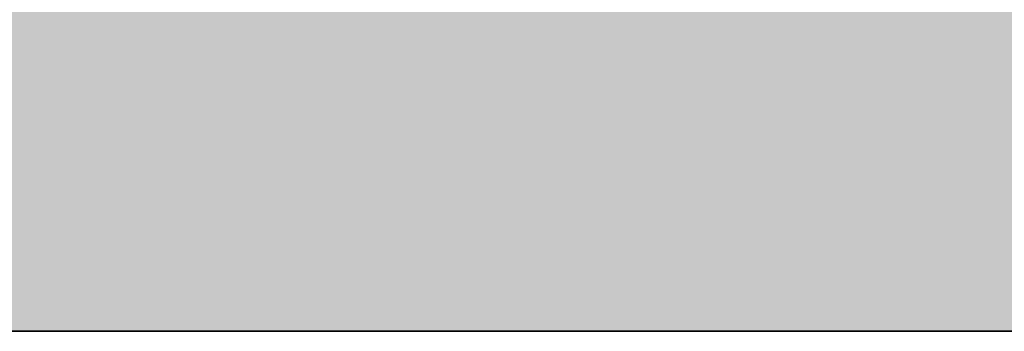
# Model space of a CAD drawing. Units: inches. Extents: x 2083 to 3317, y 1141 to 2115.
# Tile 141 of 256: x 3126.6699 to 3126.8176, y 1263.2614 to 1263.3081. Entities that reach past the tile are written whole.
import ezdxf

# ---------------------------------------------------------------- set-up
doc = ezdxf.new("R2010")
doc.units = ezdxf.units.IN
doc.layers.add('A-ANNO-DIMS', color=2, linetype='Continuous', lineweight=18)
doc.layers.add('A-WALL', color=7, linetype='Continuous', lineweight=35)
doc.layers.add('A-WALL-PATT', color=251, linetype='Continuous', lineweight=13, true_color=0x636466)
doc.styles.get("Standard").update_dxf_attribs({"font": 'arial.ttf'})
doc.dimstyles.new('ISO-25', dxfattribs={"dimtxt": 12, "dimasz": 12, "dimexe": 1.25, "dimexo": 0.625, "dimtad": 1, "dimlunit": 3, "dimtxsty": 'Standard', "dimcen": 2.5, "dimadec": 0, "dimazin": 0, "dimtfac": 1, "dimtmove": 0, "dimatfit": 3, "dimfxl": 1, "dimarcsym": 0})

# ---------------------------------------------------------------- blocks, each defined once
blk = doc.blocks.new('*D10')
at = {"layer": 'A-ANNO-DIMS', "color": 0, "lineweight": -2, "transparency": 16777216}
for p, q in [((2862.95978, 1262.63636), (2862.95978, 1201.38445)), ((3126.95978, 1262.63636), (3126.95978, 1201.38445)), ((2874.95978, 1202.63445), (3114.95978, 1202.63445))]:
    blk.add_line(p, q, dxfattribs=at)
at = {"layer": 'A-ANNO-DIMS', "color": 0, "transparency": 16777216}
for points in [[(2874.95978, 1204.63445), (2874.95978, 1200.63445), (2862.95978, 1202.63445)], [(3114.95978, 1204.63445), (3114.95978, 1200.63445), (3126.95978, 1202.63445)]]:
    blk.add_solid(points, dxfattribs=at)
at = {"layer": 'Defpoints', "color": 0, "transparency": 16777216}
for p in [(2862.95978, 1263.26136), (3126.95978, 1263.26136), (3126.95978, 1202.63445)]:
    blk.add_point(p, dxfattribs=at)
at = {"layer": 'A-ANNO-DIMS', "color": 0, "transparency": 16777216, "insert": (2994.95978, 1209.28401), "char_height": 12, "attachment_point": 5}
blk.add_mtext("22'", dxfattribs=at)
blk = doc.blocks.new('*D26')
at = {"layer": 'A-ANNO-DIMS', "color": 0, "lineweight": -2, "transparency": 16777216}
for p, q in [((3088.98584, 1274.91509), (3088.98584, 1270.95196)), ((3111.24004, 1274.91509), (3111.24004, 1270.95196)), ((3076.98584, 1272.20196), (2840.26245, 1272.20196)), ((3111.24004, 1272.20196), (3088.98584, 1272.20196)), ((3123.24004, 1272.20196), (3135.24004, 1272.20196))]:
    blk.add_line(p, q, dxfattribs=at)
at = {"layer": 'A-ANNO-DIMS', "color": 0, "transparency": 16777216}
for points in [[(3076.98584, 1274.20196), (3076.98584, 1270.20196), (3088.98584, 1272.20196)], [(3123.24004, 1274.20196), (3123.24004, 1270.20196), (3111.24004, 1272.20196)]]:
    blk.add_solid(points, dxfattribs=at)
at = {"layer": 'Defpoints', "color": 0, "transparency": 16777216}
for p in [(3088.98584, 1275.54009), (3111.24004, 1275.54009), (3088.98584, 1272.20196)]:
    blk.add_point(p, dxfattribs=at)
at = {"layer": 'A-ANNO-DIMS', "color": 0, "transparency": 16777216, "insert": (2952.62415, 1279.0316), "char_height": 12, "attachment_point": 5}
blk.add_mtext('NIGHTSTAND 1\'-10 1/2" TYP.', dxfattribs=at)
blk = doc.blocks.new('*D27')
at = {"layer": 'A-ANNO-DIMS', "color": 0, "lineweight": -2, "transparency": 16777216}
for p, q in [((3114.57817, 1309.79428), (3114.57817, 1321.79428)), ((3111.86504, 1297.79428), (3115.82817, 1297.79428)), ((3114.57817, 1297.79428), (3114.57817, 1275.54009)), ((3111.86504, 1275.54009), (3115.82817, 1275.54009)), ((3114.57817, 1263.54009), (3114.57817, 1140.98859))]:
    blk.add_line(p, q, dxfattribs=at)
at = {"layer": 'A-ANNO-DIMS', "color": 0, "transparency": 16777216}
for points in [[(3112.57817, 1309.79428), (3116.57817, 1309.79428), (3114.57817, 1297.79428)], [(3112.57817, 1263.54009), (3116.57817, 1263.54009), (3114.57817, 1275.54009)]]:
    blk.add_solid(points, dxfattribs=at)
at = {"layer": 'Defpoints', "color": 0, "transparency": 16777216}
for p in [(3111.24004, 1297.79428), (3111.24004, 1275.54009), (3114.57817, 1275.54009)]:
    blk.add_point(p, dxfattribs=at)
at = {"layer": 'A-ANNO-DIMS', "color": 0, "transparency": 16777216, "insert": (3107.74853, 1196.26434), "char_height": 12, "attachment_point": 5, "rotation": 90}
blk.add_mtext('1\'-10 1/2" TYP.', dxfattribs=at)

msp = doc.modelspace()

# ---------------------------------------------------------------- hatches: boundary and pattern name
at = {"layer": 'A-WALL-PATT'}
h = msp.add_hatch(color=256, dxfattribs=at)
h.dxf.hatch_style = 1
h.paths.add_polyline_path([(3126.95978, 2020.76136), (2748.95978, 2020.76136), (2604.95978, 2020.76136), (2226.95978, 2020.76136), (2226.95978, 1702.76136), (2466.95978, 1702.76136), (2466.95978, 1582.76136), (2418.95978, 1582.76136), (2418.95978, 1477.76136), (2226.95978, 1477.76136), (2226.95978, 1263.26136), (2544.95978, 1263.26136), (2544.95978, 1411.76136), (2604.95978, 1411.76136), (2685.95978, 1411.76136), (2685.95978, 1420.76136), (2604.95978, 1420.76136), (2604.95978, 1573.76136), (2604.95978, 1702.76136), (2604.95978, 2011.76136), (2748.95978, 2011.76136), (2748.95978, 1702.76136), (2862.95978, 1702.76136), (2862.95978, 1621.76136), (2871.95978, 1621.76136), (2871.95978, 1702.76136), (2883.95978, 1702.76136), (2883.95978, 1706.93946, -0.026459), (2883.95978, 1711.76136), (2757.95978, 1711.76136), (2757.95978, 1807.76136), (2787.95978, 1807.76136), (2787.95978, 1812.26136), (2757.95978, 1812.26136), (2757.95978, 2011.76136), (2877.95978, 2011.76136), (2877.95978, 1812.26136), (2847.95978, 1812.26136), (2847.95978, 1807.76136), (2889.83574, 1807.76136), (2889.83574, 1812.26136), (2882.45978, 1812.26136), (2882.45978, 2011.76136), (3117.95978, 2011.76136), (3117.95978, 1812.26136), (2937.83574, 1812.26136), (2937.83574, 1807.76136), (2995.70978, 1807.76136), (2995.70978, 1796.11767), (3000.20978, 1796.11767), (3000.20978, 1807.76136), (3117.95978, 1807.76136), (3117.95978, 1711.76136), (3000.20978, 1711.76136), (3000.20978, 1760.11767), (2998.5727, 1760.11767, -0.020711), (2995.70978, 1760.11767), (2995.70978, 1711.76136), (2931.95978, 1711.76136), (2931.95978, 1702.76136), (3126.95978, 1702.76136)])
h.paths.add_polyline_path([(2471.45978, 2011.76136), (2471.45978, 1810.01136), (2462.71694, 1810.01136), (2462.71694, 1805.51136), (2505.95978, 1805.51136), (2505.95978, 1810.01136), (2475.95978, 1810.01136), (2475.95978, 2011.76136), (2595.95978, 2011.76136), (2595.95978, 1810.01136), (2565.95978, 1810.01136), (2565.95978, 1805.51136), (2595.95978, 1805.51136), (2595.95978, 1711.76136), (2235.95978, 1711.76136), (2235.95978, 1805.51136), (2353.70978, 1805.51136), (2353.70978, 1796.05416), (2358.20978, 1796.05416), (2358.20978, 1805.51136), (2414.71694, 1805.51136), (2414.71694, 1810.01136), (2235.95978, 1810.01136), (2235.95978, 2011.76136)], flags=16)
h.paths.add_polyline_path([(2270.20473, 1994.61001), (2270.20473, 1970.61001), (2246.20473, 1970.61001), (2246.20473, 1994.61001)], flags=0)
edge = h.paths.add_edge_path(flags=0)
edge.add_ellipse((2332.02739, 1899.79818), major_axis=(-3.04299, 3.04299), ratio=0.1682525, start_angle=-161.33217, end_angle=-156.30711, ccw=False)
edge.add_ellipse((2333.08204, 1898.74353), major_axis=(-1.05465, 1.05465), ratio=0.4535321, start_angle=-123.37102, end_angle=-94.15911)
edge = h.paths.add_edge_path(flags=0)
edge.add_ellipse((2332.02739, 1968.87629), major_axis=(3.04299, 3.04299), ratio=0.1682525, start_angle=18.66783, end_angle=23.69289)
edge.add_spline(control_points=[(2332.9256, 1970.6911), (2332.22677, 1970.3361), (2330.89371, 1969.65891), (2328.41308, 1970.93214), (2327.20393, 1967.74871), (2324.7096, 1969.95559), (2322.53282, 1967.01235), (2320.01285, 1971.29581), (2317.68031, 1968.15784), (2316.04053, 1967.10205), (2315.4269, 1966.8096)], knot_values=[0, 0, 0, 0, 2.267059, 4.324559, 6.685584, 8.878641, 11.121502, 14.300359, 17.755284, 19.732645, 19.732645, 19.732645, 19.732645], degree=3, periodic=0)
edge.add_ellipse((2332.02739, 1968.87629), major_axis=(3.04299, 3.04299), ratio=0.1682525, start_angle=18.66783, end_angle=23.69289, ccw=False)
edge.add_ellipse((2333.08204, 1969.93094), major_axis=(1.05465, 1.05465), ratio=0.4535321, start_angle=56.62898, end_angle=85.84089, ccw=False)
edge = h.paths.add_edge_path(flags=0)
edge.add_spline(control_points=[(2296.42829, 1967.98791), (2293.6278, 1965.33631), (2287.70362, 1959.72709), (2299.74386, 1949.9957), (2294.53259, 1935.66853), (2290.57323, 1920.60351), (2293.39412, 1909.97369), (2296.18541, 1904.96654)], knot_values=[0.099185, 0.099185, 0.099185, 0.099185, 0.345301, 0.619822, 0.982653, 1.386093, 1.810555, 1.810555, 1.810555, 1.810555], degree=3, periodic=0)
edge.add_spline(control_points=[(2296.18541, 1904.96654), (2297.38358, 1902.6193), (2298.00097, 1901.94931), (2298.55297, 1901.46815)], knot_values=[0.006246, 0.006246, 0.006246, 0.006246, 0.055476, 0.055476, 0.055476, 0.055476], degree=3, periodic=0)
edge.add_spline(control_points=[(2298.55297, 1901.46815), (2297.25861, 1900.92322), (2295.22529, 1900.23213), (2293.06023, 1900.61421), (2292.10142, 1900.78841), (2292.08958, 1900.79057)], knot_values=[0.312835, 0.312835, 0.312835, 0.312835, 0.40178, 0.474987, 0.475903, 0.475903, 0.475903, 0.475903], degree=3, periodic=0)
edge.add_arc((2292.79365, 1904.66411), 3.93701, 215.4209, 259.69818, ccw=False)
edge.add_spline(control_points=[(2289.58531, 1902.3823), (2289.47665, 1902.53509), (2289.36848, 1902.68804), (2289.26086, 1902.84117)], knot_values=[0.102872, 0.102872, 0.102872, 0.102872, 0.116896, 0.116896, 0.116896, 0.116896], degree=3, periodic=0)
edge.add_spline(control_points=[(2289.26086, 1902.84117), (2288.6866, 1902.55019), (2287.64005, 1902.0199), (2285.88134, 1901.87395), (2283.85297, 1901.50435), (2281.71999, 1899.71054), (2278.46699, 1899.49294), (2276.15714, 1901.8832), (2272.25895, 1899.80407), (2267.77761, 1901.84318), (2262.24388, 1900.18403), (2257.41493, 1901.78206), (2254.31837, 1900.72612), (2253.17828, 1900.33734)], knot_values=[0, 0, 0, 0, 1.907977, 3.477176, 5.261074, 7.972851, 11.680248, 13.717921, 16.939592, 22.789562, 27.502503, 33.595215, 37.145618, 37.145618, 37.145618, 37.145618], degree=3, periodic=0)
edge.add_line((2253.17828, 1900.33734), (2250.24424, 1902.84117))
edge.add_line((2250.24424, 1902.84117), (2250.24424, 1965.8333))
edge.add_line((2250.24424, 1965.8333), (2253.17828, 1968.33712))
edge.add_spline(control_points=[(2253.17828, 1968.33712), (2254.31837, 1967.94835), (2257.41493, 1966.89241), (2262.24388, 1968.49043), (2267.77761, 1966.83128), (2271.52673, 1968.53722), (2273.87591, 1967.82829), (2274.2067, 1967.72764)], knot_values=[0, 0, 0, 0, 0.09018, 0.244935, 0.364644, 0.513233, 0.537855, 0.537855, 0.537855, 0.537855], degree=3, periodic=0)
edge.add_arc((2274.35289, 1963.79335), 3.93701, 72.05113, 92.12795, ccw=False)
edge.add_arc((2281.29693, 1985.23), 18.5963, 252.051134, 288.565722)
edge.add_arc((2292.31672, 1956.02888), 12.64608, 71.026788, 113.778218, ccw=False)
edge = h.paths.add_edge_path(flags=0)
edge.add_spline(control_points=[(2274.89941, 1951.85619), (2275.06616, 1951.61659), (2275.23269, 1951.37659), (2275.39799, 1951.13585)], knot_values=[1.409916, 1.409916, 1.409916, 1.409916, 1.43159, 1.43159, 1.43159, 1.43159], degree=3, periodic=0)
edge.add_spline(control_points=[(2275.39799, 1951.13585), (2275.79211, 1950.56189), (2276.17923, 1949.98377), (2276.54555, 1949.3971)], knot_values=[1.358238, 1.358238, 1.358238, 1.358238, 1.409916, 1.409916, 1.409916, 1.409916], degree=3, periodic=0)
edge.add_line((2276.54555, 1949.3971), (2277.43729, 1947.86218))
edge.add_spline(control_points=[(2277.43729, 1947.86218), (2276.30383, 1945.67311), (2274.6397, 1942.42688), (2274.63161, 1938.0939), (2272.79912, 1930.85155), (2274.35643, 1943.89705), (2275.94768, 1947.92336), (2276.54555, 1949.3971)], knot_values=[0.005632, 0.005632, 0.005632, 0.005632, 0.186014, 0.266002, 0.357087, 0.59639, 0.739732, 0.739732, 0.739732, 0.739732], degree=3, periodic=0)
edge.add_spline(control_points=[(2276.54555, 1949.3971), (2276.17923, 1949.98377), (2275.79211, 1950.56189), (2275.39799, 1951.13585)], knot_values=[1.358238, 1.358238, 1.358238, 1.358238, 1.409916, 1.409916, 1.409916, 1.409916], degree=3, periodic=0)
edge.add_spline(control_points=[(2275.39799, 1951.13585), (2274.9425, 1950.08045), (2274.20776, 1948.02527), (2273.9346, 1944.85148), (2272.46853, 1937.62749), (2273.46622, 1945.69647), (2274.70062, 1951.05947), (2274.89941, 1951.85619)], knot_values=[0.104364, 0.104364, 0.104364, 0.104364, 0.189636, 0.269624, 0.36071, 0.600013, 0.644622, 0.644622, 0.644622, 0.644622], degree=3, periodic=0)
h.paths.add_polyline_path([(2269.16751, 1963.12757, -0.357527), (2268.17063, 1960.97637, -0.092561), (2268.17063, 1939.43632, -0.357527), (2269.16751, 1937.28512, -0.357527), (2267.01631, 1938.282, -0.164785), (2254.68558, 1938.282, -0.357527), (2252.53438, 1937.28512, -0.357527), (2253.53126, 1939.43632, -0.092561), (2253.53126, 1960.97637, -0.357527), (2252.53438, 1963.12757, -0.357527), (2254.68558, 1962.13069, -0.164785), (2267.01631, 1962.13069, -0.357527)], flags=0)
h.paths.add_polyline_path([(2248.87407, 1967.8018), (2248.87407, 1957.02771), (2249.45778, 1957.02771), (2249.45778, 1911.64676), (2248.87407, 1911.64676), (2248.87407, 1900.87267), (2246.51186, 1900.87267, 0.197327), (2244.14966, 1902.45687), (2244.14966, 1966.21759, 0.197327), (2246.51186, 1967.8018)], flags=0)
h.paths.add_polyline_path([(2269.16751, 1931.38934, -0.357527), (2268.17063, 1929.23814, -0.092561), (2268.17063, 1907.6981, -0.357527), (2269.16751, 1905.54689, -0.357527), (2267.01631, 1906.54377, -0.164785), (2254.68558, 1906.54377, -0.357527), (2252.53438, 1905.54689, -0.357527), (2253.53126, 1907.6981, -0.092561), (2253.53126, 1929.23814, -0.357527), (2252.53438, 1931.38934, -0.357527), (2254.68558, 1930.39246, -0.164785), (2267.01631, 1930.39246, -0.357527)], flags=0)
edge = h.paths.add_edge_path(flags=0)
edge.add_spline(control_points=[(2276.19686, 1906.7237), (2276.16814, 1909.02893), (2276.11405, 1913.37185), (2270.59842, 1924.92498), (2273.90517, 1919.01278), (2275.92171, 1916.26206), (2275.47457, 1912.40215), (2277.25787, 1910.38062), (2276.69604, 1908.22504), (2276.64622, 1906.81302), (2276.61782, 1906.00841)], knot_values=[0, 0, 0, 0, 8.61026, 16.221274, 18.843057, 23.804898, 27.440828, 29.356102, 31.203478, 33.650687, 33.650687, 33.650687, 33.650687], degree=3, periodic=0)
edge.add_spline(control_points=[(2276.61782, 1906.00841), (2276.62331, 1905.62414), (2276.49774, 1904.62866), (2275.44178, 1903.85473), (2274.93731, 1903.08045), (2274.85908, 1902.84117)], knot_values=[0.156488, 0.156488, 0.156488, 0.156488, 0.184398, 0.231376, 0.250598, 0.250598, 0.250598, 0.250598], degree=3, periodic=0)
edge.add_line((2274.85908, 1902.84117), (2276.50598, 1902.84117))
edge.add_spline(control_points=[(2276.50598, 1902.84117), (2276.78831, 1903.08494), (2277.66507, 1904.1252), (2278.24954, 1904.34074), (2277.65387, 1908.52739), (2278.15567, 1906.22781), (2278.10046, 1905.28595), (2278.84667, 1904.06901), (2277.85679, 1903.41495), (2277.87419, 1902.99105), (2277.90356, 1902.84117)], knot_values=[0.059574, 0.059574, 0.059574, 0.059574, 0.080753, 0.103741, 0.16972, 0.176036, 0.207137, 0.240474, 0.262341, 0.27366, 0.27366, 0.27366, 0.27366], degree=3, periodic=0)
edge.add_line((2277.90356, 1902.84117), (2280.02983, 1902.84117))
edge.add_spline(control_points=[(2280.02983, 1902.84117), (2279.88822, 1903.0884), (2279.49926, 1903.98155), (2280.15228, 1905.93935), (2278.10362, 1909.65776), (2279.76239, 1907.18529), (2280.3279, 1904.87486), (2280.48511, 1903.48959), (2281.46327, 1903.24943), (2281.75834, 1902.9365), (2281.83404, 1902.84117)], knot_values=[0.013856, 0.013856, 0.013856, 0.013856, 0.034874, 0.088867, 0.107879, 0.126738, 0.158714, 0.193757, 0.217487, 0.226722, 0.226722, 0.226722, 0.226722], degree=3, periodic=0)
edge.add_spline(control_points=[(2281.83404, 1902.84117), (2281.78753, 1902.8267), (2281.64702, 1902.78299), (2281.39553, 1902.85949), (2281.08808, 1902.98524), (2280.72068, 1903.0609), (2280.33345, 1903.02573), (2280.12477, 1902.89888), (2280.02983, 1902.84117)], knot_values=[0, 0, 0, 0, 0.14413, 0.435517, 0.749276, 1.153046, 1.548371, 1.878348, 1.878348, 1.878348, 1.878348], degree=3, periodic=0)
edge.add_line((2280.02983, 1902.84117), (2277.90356, 1902.84117))
edge.add_spline(control_points=[(2277.90356, 1902.84117), (2277.89286, 1902.79586), (2277.8654, 1902.67964), (2277.60748, 1902.68748), (2277.27405, 1902.8007), (2276.83792, 1902.61977), (2276.58381, 1902.78926), (2276.50598, 1902.84117)], knot_values=[0, 0, 0, 0, 0.127189, 0.326199, 0.628009, 1.24357, 1.515331, 1.515331, 1.515331, 1.515331], degree=3, periodic=0)
edge.add_line((2276.50598, 1902.84117), (2274.85908, 1902.84117))
edge.add_spline(control_points=[(2274.85908, 1902.84117), (2274.81444, 1902.89859), (2274.72513, 1903.01345), (2274.49348, 1903.11897), (2274.24429, 1902.96054), (2273.93712, 1903.18494), (2273.61404, 1902.98314), (2273.40832, 1902.88304), (2273.32225, 1902.84117)], knot_values=[0, 0, 0, 0, 0.21843, 0.436957, 0.687977, 0.990379, 1.398396, 1.69185, 1.69185, 1.69185, 1.69185], degree=3, periodic=0)
edge.add_spline(control_points=[(2273.32225, 1902.84117), (2273.61674, 1903.44569), (2274.274, 1904.53825), (2276.02724, 1904.5737), (2276.20696, 1906.58364), (2276.19686, 1906.7237)], knot_values=[0.012227, 0.012227, 0.012227, 0.012227, 0.059472, 0.106218, 0.134458, 0.134458, 0.134458, 0.134458], degree=3, periodic=0)
h.paths.add_polyline_path([(2270.77605, 1897.78983), (2270.77605, 1873.78983), (2246.77605, 1873.78983), (2246.77605, 1897.78983)], flags=0)
h.paths.add_polyline_path([(2353.70978, 1760.00506), (2353.70978, 1760.05416), (2358.20978, 1760.05416, -0.033729)], flags=0)
h.paths.add_polyline_path([(2321.81912, 1737.52919), (2341.99533, 1737.52919, -0.414214), (2343.20327, 1736.32124), (2343.20327, 1721.0206, -0.414214), (2341.99533, 1719.81265), (2321.81912, 1719.81265, -0.414214), (2320.61117, 1721.0206), (2320.61117, 1736.32124, -0.414214)], flags=0)
h.paths.add_polyline_path([(2324.23501, 1736.32124), (2339.57944, 1736.32124, -0.414214), (2341.99533, 1733.90535), (2341.99533, 1725.44973, -0.414214), (2339.57944, 1723.03384), (2333.68059, 1723.03384), (2333.84532, 1722.04547, -0.870646), (2335.4254, 1721.82589, -0.767327), (2333.92269, 1721.42324), (2331.29102, 1721.42324, -0.767327), (2329.78832, 1721.82589, -0.870646), (2331.3684, 1722.04547), (2331.53313, 1723.03384), (2324.23501, 1723.03384, -0.414214), (2321.81912, 1725.44973), (2321.81912, 1733.90535, -0.414214)], flags=0)
h.paths.add_polyline_path([(2570.48379, 1928.61544), (2589.68379, 1928.61544), (2590.16883, 1928.61544), (2590.16883, 1904.9934), (2570.48379, 1904.9934)], flags=0)
h.paths.add_polyline_path([(2574.44732, 1927.26382, -1), (2572.82884, 1927.26382, -1)], flags=0)
h.paths.add_polyline_path([(2573.08987, 1926.94088), (2573.92503, 1927.77604), (2574.14774, 1927.55333), (2573.31258, 1926.71817)], flags=0)
h.paths.add_polyline_path([(2578.77906, 1919.72962, -1), (2571.59166, 1919.72962, -1)], flags=0)
h.paths.add_polyline_path([(2578.38536, 1919.72962, -1), (2571.98536, 1919.72962, -1)], flags=0)
h.paths.add_polyline_path([(2331.59576, 1729.47622, -1), (2333.61795, 1729.47622, -1)], flags=0)
h.paths.add_polyline_path([(2578.03423, 1927.26382, -1), (2576.41574, 1927.26382, -1)], flags=0)
h.paths.add_polyline_path([(2576.68885, 1927.53109), (2576.91156, 1927.7538), (2577.74673, 1926.91863), (2577.52402, 1926.69592)], flags=0)
h.paths.add_polyline_path([(2578.13906, 1909.85954, -1), (2572.23166, 1909.85954, -1)], flags=0)
h.paths.add_polyline_path([(2577.74536, 1909.85954, -1), (2572.62536, 1909.85954, -1)], flags=0)
h.paths.add_polyline_path([(2583.79772, 1927.26382, -1), (2582.17923, 1927.26382, -1)], flags=0)
h.paths.add_polyline_path([(2582.71865, 1927.7538), (2583.55381, 1926.91863), (2583.3311, 1926.69592), (2582.49594, 1927.53109)], flags=0)
h.paths.add_polyline_path([(2582.49594, 1927.53109), (2582.71865, 1927.7538), (2583.55381, 1926.91863), (2583.3311, 1926.69592)], flags=0)
h.paths.add_polyline_path([(2587.73906, 1920.52962, -1), (2581.83166, 1920.52962, -1)], flags=0)
h.paths.add_polyline_path([(2587.34536, 1920.52962, -1), (2582.22536, 1920.52962, -1)], flags=0)
h.paths.add_polyline_path([(2587.38462, 1927.26382, -1), (2585.76613, 1927.26382, -1)], flags=0)
h.paths.add_polyline_path([(2586.08199, 1926.98025), (2586.91716, 1927.81541), (2587.13987, 1927.5927), (2586.3047, 1926.75754)], flags=0)
h.paths.add_polyline_path([(2588.37906, 1910.65954, -1), (2581.19166, 1910.65954, -1)], flags=0)
h.paths.add_polyline_path([(2587.98536, 1910.65954, -1), (2581.58536, 1910.65954, -1)], flags=0)
h.paths.add_polyline_path([(2417.16773, 1729.4779), (2437.34394, 1729.4779, -0.414214), (2438.55188, 1728.26995), (2438.55188, 1712.96931, -0.414214), (2437.34394, 1711.76136), (2417.16773, 1711.76136, -0.414214), (2415.95978, 1712.96931), (2415.95978, 1728.26995, -0.414214)], flags=0)
h.paths.add_polyline_path([(2419.58362, 1728.26995), (2434.92805, 1728.26995, -0.414214), (2437.34394, 1725.85406), (2437.34394, 1717.39844, -0.414214), (2434.92805, 1714.98255), (2429.0292, 1714.98255), (2429.19393, 1713.99418, -0.870646), (2430.77401, 1713.7746, -0.767327), (2429.2713, 1713.37195), (2426.63963, 1713.37195, -0.767327), (2425.13693, 1713.7746, -0.870646), (2426.71701, 1713.99418), (2426.88174, 1714.98255), (2419.58362, 1714.98255, -0.414214), (2417.16773, 1717.39844), (2417.16773, 1725.85406, -0.414214)], flags=0)
h.paths.add_polyline_path([(2419.58362, 1728.26995), (2434.92805, 1728.26995, -0.414214), (2437.34394, 1725.85406), (2437.34394, 1717.39844, -0.414214), (2434.92805, 1714.98255), (2429.0292, 1714.98255), (2428.35812, 1719.00903), (2427.55282, 1719.00903), (2426.88174, 1714.98255), (2419.58362, 1714.98255, -0.414214), (2417.16773, 1717.39844), (2417.16773, 1725.85406, -0.414214)], flags=0)
h.paths.add_polyline_path([(2426.94437, 1721.42492, -1), (2428.96656, 1721.42492, -1)], flags=0)
h.paths.add_polyline_path([(2475.95978, 1702.76136), (2595.95978, 1702.76136), (2595.95978, 1582.76136), (2475.95978, 1582.76136)], flags=16)
h.paths.add_polyline_path([(2427.95978, 1573.76136), (2595.95978, 1573.76136), (2595.95978, 1468.76136), (2595.95978, 1420.76136), (2384.45978, 1420.76136), (2384.45978, 1468.76136), (2427.95978, 1468.76136)], flags=16)
h.paths.add_polyline_path([(2379.95978, 1468.76136), (2379.95978, 1420.76136), (2235.95978, 1420.76136), (2235.95978, 1468.76136)], flags=16)
h.paths.add_polyline_path([(2317.816, 1466.69577), (2337.9922, 1466.69577, -0.414214), (2339.20015, 1465.48782), (2339.20015, 1450.18718, -0.414214), (2337.9922, 1448.97923), (2317.816, 1448.97923, -0.414214), (2316.60805, 1450.18718), (2316.60805, 1465.48782, -0.414214)], flags=0)
h.paths.add_polyline_path([(2320.23189, 1465.48782), (2335.57631, 1465.48782, -0.414214), (2337.9922, 1463.07193), (2337.9922, 1454.61631, -0.414214), (2335.57631, 1452.20042), (2329.67747, 1452.20042), (2329.84219, 1451.21205, -0.870646), (2331.42228, 1450.99247, -0.767327), (2329.91957, 1450.58983), (2327.2879, 1450.58983, -0.767327), (2325.7852, 1450.99247, -0.870646), (2327.36528, 1451.21205), (2327.53001, 1452.20042), (2320.23189, 1452.20042, -0.414214), (2317.816, 1454.61631), (2317.816, 1463.07193, -0.414214)], flags=0)
h.paths.add_polyline_path([(2320.23189, 1465.48782), (2335.57631, 1465.48782, -0.414214), (2337.9922, 1463.07193), (2337.9922, 1454.61631, -0.414214), (2335.57631, 1452.20042), (2329.67747, 1452.20042), (2329.00638, 1456.22691), (2328.20109, 1456.22691), (2327.53001, 1452.20042), (2320.23189, 1452.20042, -0.414214), (2317.816, 1454.61631), (2317.816, 1463.07193, -0.414214)], flags=0)
h.paths.add_polyline_path([(2327.59264, 1458.6428, -1), (2329.61483, 1458.6428, -1)], flags=0)
h.paths.add_polyline_path([(2244.41174, 1433.34045), (2241.92094, 1433.34045, -0.414214), (2240.01786, 1435.24354), (2240.01786, 1440.95281, -0.414211), (2241.92093, 1442.8559), (2244.41174, 1442.8559, -1.976472)], flags=0)
h.paths.add_polyline_path([(2245.35689, 1434.39754, -0.414214), (2245.35689, 1441.79881, -2.144098)], flags=0)
h.paths.add_polyline_path([(2535.95978, 1416.26136), (2535.95978, 1272.26136), (2235.95978, 1272.26136), (2235.95978, 1416.26136)], flags=16)
h.paths.add_polyline_path([(2260.11956, 1384.29284), (2260.11956, 1362.03865), (2237.86537, 1362.03865), (2237.86537, 1384.29284)], flags=0)
edge = h.paths.add_edge_path(flags=0)
edge.add_line((2318.25185, 1362.0933), (2318.1458, 1362.00097))
edge.add_ellipse((2317.44512, 1360.43104), major_axis=(2.82164, 2.82164), ratio=0.1682525, start_angle=18.66783, end_angle=20.94813, ccw=False)
edge.add_ellipse((2318.42305, 1361.40897), major_axis=(0.97793, 0.97793), ratio=0.4535321, start_angle=56.62898, end_angle=70.2262, ccw=False)
edge = h.paths.add_edge_path(flags=0)
edge.add_line((2319.10737, 1295.57108), (2319.01504, 1295.67713))
edge.add_ellipse((2317.44512, 1296.37781), major_axis=(-2.82164, 2.82164), ratio=0.1682525, start_angle=-161.33217, end_angle=-159.05187, ccw=False)
edge.add_ellipse((2318.42305, 1295.39988), major_axis=(-0.97793, 0.97793), ratio=0.4535321, start_angle=-123.37102, end_angle=-109.7738)
edge = h.paths.add_edge_path(flags=0)
edge.add_spline(control_points=[(2284.21035, 1301.17022), (2284.58069, 1300.44472), (2284.89119, 1299.89202), (2285.15955, 1299.46102)], knot_values=[0.039066, 0.039066, 0.039066, 0.039066, 0.055476, 0.055476, 0.055476, 0.055476], degree=3, periodic=0)
edge.add_line((2285.15955, 1299.46102), (2284.21035, 1301.17022))
edge = h.paths.add_edge_path(flags=0)
edge.add_line((2280.41246, 1297.29801), (2283.36999, 1297.03612))
edge.add_line((2283.36999, 1297.03612), (2286.40569, 1297.92631))
edge.add_spline(control_points=[(2286.40569, 1297.92631), (2285.30549, 1297.46312), (2284.34478, 1297.12915), (2283.36999, 1297.03612)], knot_values=[0.394369, 0.394369, 0.394369, 0.394369, 0.475903, 0.475903, 0.475903, 0.475903], degree=3, periodic=0)
edge.add_spline(control_points=[(2283.36999, 1297.03612), (2283.28139, 1297.02767), (2282.31629, 1296.95734), (2281.3125, 1297.13448), (2280.42344, 1297.29602), (2280.41246, 1297.29801)], knot_values=[0.312835, 0.312835, 0.312835, 0.312835, 0.320246, 0.393453, 0.394369, 0.394369, 0.394369, 0.394369], degree=3, periodic=0)
edge = h.paths.add_edge_path(flags=0)
edge.add_line((2284.43556, 1359.60729), (2280.44629, 1355.32805))
edge.add_line((2280.44629, 1355.32805), (2279.57999, 1351.01775))
edge.add_line((2279.57999, 1351.01775), (2282.41297, 1346.58043))
edge.add_spline(control_points=[(2282.41297, 1346.58043), (2283.15333, 1345.58924), (2284.2529, 1344.0289), (2284.80104, 1342.38717), (2284.93516, 1341.80554)], knot_values=[1.240098, 1.240098, 1.240098, 1.240098, 1.332892, 1.382712, 1.382712, 1.382712, 1.382712], degree=3, periodic=0)
edge.add_spline(control_points=[(2284.93516, 1341.80554), (2285.31911, 1340.1406), (2285.23303, 1338.4092), (2284.90994, 1336.65412)], knot_values=[1.097484, 1.097484, 1.097484, 1.097484, 1.240098, 1.240098, 1.240098, 1.240098], degree=3, periodic=0)
edge.add_spline(control_points=[(2284.90994, 1336.65412), (2284.58685, 1334.89904), (2284.02675, 1333.12027), (2283.46264, 1331.36058)], knot_values=[0.95487, 0.95487, 0.95487, 0.95487, 1.097484, 1.097484, 1.097484, 1.097484], degree=3, periodic=0)
edge.add_line((2283.46264, 1331.36058), (2281.89038, 1326.15336))
edge.add_line((2281.89038, 1326.15336), (2280.75626, 1321.05609))
edge.add_line((2280.75626, 1321.05609), (2280.2992, 1316.00198))
edge.add_line((2280.2992, 1316.00198), (2280.71593, 1310.95007))
edge.add_line((2280.71593, 1310.95007), (2282.02809, 1305.97214))
edge.add_line((2282.02809, 1305.97214), (2284.21035, 1301.17022))
edge.add_spline(control_points=[(2284.21035, 1301.17022), (2283.34073, 1302.73019), (2282.6119, 1304.33649), (2282.02809, 1305.97214)], knot_values=[0.099185, 0.099185, 0.099185, 0.099185, 0.241799, 0.241799, 0.241799, 0.241799], degree=3, periodic=0)
edge.add_spline(control_points=[(2282.02809, 1305.97214), (2281.44428, 1307.60778), (2281.00549, 1309.27276), (2280.71593, 1310.95007)], knot_values=[0.241799, 0.241799, 0.241799, 0.241799, 0.384413, 0.384413, 0.384413, 0.384413], degree=3, periodic=0)
edge.add_spline(control_points=[(2280.71593, 1310.95007), (2280.43324, 1312.58761), (2280.28939, 1314.27696), (2280.29889, 1315.96203), (2280.2992, 1316.00198)], knot_values=[0.384413, 0.384413, 0.384413, 0.384413, 0.523647, 0.527028, 0.527028, 0.527028, 0.527028], degree=3, periodic=0)
edge.add_spline(control_points=[(2280.2992, 1316.00198), (2280.31233, 1317.68696), (2280.47787, 1319.36793), (2280.75626, 1321.05609)], knot_values=[0.527028, 0.527028, 0.527028, 0.527028, 0.669642, 0.669642, 0.669642, 0.669642], degree=3, periodic=0)
edge.add_spline(control_points=[(2280.75626, 1321.05609), (2281.03465, 1322.74425), (2281.42588, 1324.43961), (2281.89038, 1326.15336)], knot_values=[0.669642, 0.669642, 0.669642, 0.669642, 0.812256, 0.812256, 0.812256, 0.812256], degree=3, periodic=0)
edge.add_spline(control_points=[(2281.89038, 1326.15336), (2282.26438, 1327.53325), (2282.78787, 1329.26181), (2283.35275, 1331.01778), (2283.46264, 1331.36058)], knot_values=[0.812256, 0.812256, 0.812256, 0.812256, 0.927087, 0.95487, 0.95487, 0.95487, 0.95487], degree=3, periodic=0)
edge.add_line((2283.46264, 1331.36058), (2284.90994, 1336.65412))
edge.add_line((2284.90994, 1336.65412), (2284.93516, 1341.80554))
edge.add_line((2284.93516, 1341.80554), (2282.41297, 1346.58043))
edge.add_spline(control_points=[(2282.41297, 1346.58043), (2281.27513, 1348.10379), (2280.07845, 1349.57032), (2279.57999, 1351.01775)], knot_values=[1.382712, 1.382712, 1.382712, 1.382712, 1.525326, 1.525326, 1.525326, 1.525326], degree=3, periodic=0)
edge.add_spline(control_points=[(2279.57999, 1351.01775), (2279.44328, 1351.41472), (2279.13631, 1352.85692), (2279.73519, 1354.29039), (2280.44629, 1355.32805)], knot_values=[1.525326, 1.525326, 1.525326, 1.525326, 1.564439, 1.667941, 1.667941, 1.667941, 1.667941], degree=3, periodic=0)
edge.add_spline(control_points=[(2280.44629, 1355.32805), (2281.42611, 1356.75784), (2282.93084, 1358.18256), (2284.43556, 1359.60729)], knot_values=[1.667941, 1.667941, 1.667941, 1.667941, 1.810555, 1.810555, 1.810555, 1.810555], degree=3, periodic=0)
edge.add_arc((2280.62307, 1348.51818), 11.72618, 71.026788, 113.778218)
edge.add_arc((2270.40489, 1375.59516), 17.24357, 252.051134, 288.565722, ccw=False)
edge.add_arc((2263.96597, 1355.71785), 3.65062, 72.05113, 92.12795)
edge.add_arc((2263.96597, 1355.71785), 3.65062, 92.12795, 177.98513)
edge.add_spline(control_points=[(2260.3176, 1355.8462), (2260.26042, 1354.22067), (2260.55128, 1350.18655), (2262.99934, 1346.76625), (2264.47274, 1344.64902)], knot_values=[1.43159, 1.43159, 1.43159, 1.43159, 1.564144, 1.770695, 1.770695, 1.770695, 1.770695], degree=3, periodic=0)
edge.add_line((2264.47274, 1344.64902), (2264.93559, 1343.98253))
edge.add_spline(control_points=[(2263.80104, 1340.24811), (2263.84324, 1340.51409), (2264.06724, 1341.75647), (2264.51269, 1343.00245), (2264.93505, 1343.98108)], knot_values=[0.53657, 0.53657, 0.53657, 0.53657, 0.559349, 0.644622, 0.644622, 0.644622, 0.644622], degree=3, periodic=0)
edge.add_spline(control_points=[(2264.93505, 1343.98108), (2265.11777, 1343.71497), (2265.29888, 1343.44791), (2265.47676, 1343.17936)], knot_values=[1.384077, 1.384077, 1.384077, 1.384077, 1.409916, 1.409916, 1.409916, 1.409916], degree=3, periodic=0)
edge.add_spline(control_points=[(2265.47676, 1343.17936), (2265.65464, 1342.91082), (2265.8293, 1342.64081), (2265.99913, 1342.36881)], knot_values=[1.358238, 1.358238, 1.358238, 1.358238, 1.384077, 1.384077, 1.384077, 1.384077], degree=3, periodic=0)
edge.add_line((2265.99913, 1342.36881), (2266.82601, 1340.94555))
edge.add_spline(control_points=[(2266.82601, 1340.94555), (2268.8944, 1337.08969), (2271.39817, 1325.843), (2270.51616, 1310.56856), (2275.91938, 1301.86061), (2277.78951, 1299.19945)], knot_values=[0.116896, 0.116896, 0.116896, 0.116896, 0.472987, 1.050969, 1.313793, 1.313793, 1.313793, 1.313793], degree=3, periodic=0)
edge.add_spline(control_points=[(2277.78951, 1299.19945), (2277.83941, 1299.12845), (2277.88943, 1299.0575), (2277.93957, 1298.98658)], knot_values=[0.109884, 0.109884, 0.109884, 0.109884, 0.116896, 0.116896, 0.116896, 0.116896], degree=3, periodic=0)
edge.add_line((2277.93957, 1298.98658), (2277.78885, 1299.19911))
edge.add_spline(control_points=[(2277.78885, 1299.19911), (2277.25658, 1298.92941), (2276.28635, 1298.4379), (2275.03935, 1298.33442), (2274.38333, 1298.2389), (2274.21525, 1298.20934)], knot_values=[33.12187, 33.12187, 33.12187, 33.12187, 35.029056, 36.598255, 37.144827, 37.144827, 37.144827, 37.144827], degree=3, periodic=0)
edge.add_line((2274.21525, 1298.20934), (2273.07315, 1297.89296))
edge.add_spline(control_points=[(2273.07315, 1297.89296), (2272.32294, 1297.57978), (2271.03915, 1296.51051), (2269.24839, 1296.22606), (2268.4231, 1296.37465)], knot_values=[26.532584, 26.532584, 26.532584, 26.532584, 29.198919, 31.839101, 31.839101, 31.839101, 31.839101], degree=3, periodic=0)
edge.add_line((2268.4231, 1296.37465), (2263.8785, 1297.45753))
edge.add_spline(control_points=[(2263.8785, 1297.45753), (2263.55608, 1297.35943), (2261.86031, 1296.83869), (2260.23878, 1297.28241), (2258.93345, 1297.51646)], knot_values=[15.919551, 15.919551, 15.919551, 15.919551, 16.939592, 21.226067, 21.226067, 21.226067, 21.226067], degree=3, periodic=0)
edge.add_line((2258.93345, 1297.51646), (2254.05523, 1297.32901))
edge.add_spline(control_points=[(2254.05523, 1297.32901), (2253.75553, 1297.29582), (2252.11368, 1297.16517), (2250.46187, 1297.54422), (2249.12969, 1297.66788)], knot_values=[5.306517, 5.306517, 5.306517, 5.306517, 6.276435, 10.613034, 10.613034, 10.613034, 10.613034], degree=3, periodic=0)
edge.add_line((2249.12969, 1297.66788), (2244.33165, 1296.87776))
edge.add_line((2244.33165, 1296.87776), (2241.61103, 1299.19945))
edge.add_line((2241.61103, 1299.19945), (2241.61103, 1357.6094))
edge.add_line((2241.61103, 1357.6094), (2244.33165, 1359.9311))
edge.add_line((2244.33165, 1359.9311), (2252.72882, 1359.54269))
edge.add_spline(control_points=[(2252.72882, 1359.54269), (2252.87094, 1359.54644), (2253.30574, 1359.54817), (2253.73984, 1359.51427), (2254.03174, 1359.48243)], knot_values=[0.233291, 0.233291, 0.233291, 0.233291, 0.244935, 0.268927, 0.268927, 0.268927, 0.268927], degree=3, periodic=0)
edge.add_line((2254.03174, 1359.48243), (2259.58719, 1359.41639))
edge.add_spline(control_points=[(2259.58719, 1359.41639), (2260.67707, 1359.6285), (2262.0732, 1359.897), (2263.52369, 1359.45928), (2263.83042, 1359.36595)], knot_values=[0.422516, 0.422516, 0.422516, 0.422516, 0.513233, 0.537855, 0.537855, 0.537855, 0.537855], degree=3, periodic=0)
edge.add_arc((2263.96597, 1355.71785), 3.65062, 72.05113, 92.12795, ccw=False)
edge.add_arc((2270.40489, 1375.59516), 17.24357, 252.051134, 288.565722)
edge.add_arc((2280.62307, 1348.51818), 11.72618, 71.026788, 113.778218, ccw=False)
h.paths.add_polyline_path([(2240.34053, 1359.43471), (2240.34053, 1349.44435), (2240.88178, 1349.44435), (2240.88178, 1307.3645), (2240.34053, 1307.3645), (2240.34053, 1297.37414), (2238.15016, 1297.37414, 0.197327), (2235.95978, 1298.84311), (2235.95978, 1357.96575, 0.197327), (2238.15016, 1359.43471)], flags=0)
h.paths.add_polyline_path([(2259.15779, 1355.1005, -0.357527), (2258.23342, 1353.10578, -0.092561), (2258.23342, 1333.1326, -0.357527), (2259.15779, 1331.13788, -0.357527), (2257.16307, 1332.06225, -0.164785), (2245.7293, 1332.06225, -0.357527), (2243.73458, 1331.13788, -0.357527), (2244.65895, 1333.1326, -0.092561), (2244.65895, 1353.10578, -0.357527), (2243.73458, 1355.1005, -0.357527), (2245.7293, 1354.17613, -0.164785), (2257.16307, 1354.17613, -0.357527)], flags=0)
edge = h.paths.add_edge_path(flags=0)
edge.add_line((2265.99913, 1342.36881), (2266.82601, 1340.94555))
edge.add_line((2266.82601, 1340.94555), (2265.30756, 1337.81407))
edge.add_line((2265.30756, 1337.81407), (2264.35823, 1334.65294))
edge.add_line((2264.35823, 1334.65294), (2264.26201, 1333.7997))
edge.add_spline(control_points=[(2264.26201, 1333.7997), (2264.20836, 1333.18705), (2264.16206, 1332.36553), (2264.00714, 1331.41393), (2263.96905, 1331.20183)], knot_values=[0.464444, 0.464444, 0.464444, 0.464444, 0.516691, 0.531608, 0.531608, 0.531608, 0.531608], degree=3, periodic=0)
edge.add_spline(control_points=[(2263.96905, 1331.20183), (2263.77453, 1330.11887), (2263.42437, 1328.79084), (2263.25742, 1328.53065), (2263.23403, 1328.51461)], knot_values=[0.372682, 0.372682, 0.372682, 0.372682, 0.44885, 0.464444, 0.464444, 0.464444, 0.464444], degree=3, periodic=0)
edge.add_spline(control_points=[(2263.23403, 1328.51461), (2263.09638, 1328.42023), (2263.13117, 1329.30148), (2263.27495, 1330.61575)], knot_values=[0.280919, 0.280919, 0.280919, 0.280919, 0.372682, 0.372682, 0.372682, 0.372682], degree=3, periodic=0)
edge.add_spline(control_points=[(2263.27495, 1330.61575), (2263.41874, 1331.93002), (2263.67152, 1333.67732), (2263.96985, 1335.31503)], knot_values=[0.189157, 0.189157, 0.189157, 0.189157, 0.280919, 0.280919, 0.280919, 0.280919], degree=3, periodic=0)
edge.add_spline(control_points=[(2263.96985, 1335.31503), (2264.1005, 1336.03219), (2264.41878, 1337.62191), (2264.75485, 1338.86443), (2264.94742, 1339.49112)], knot_values=[0.097394, 0.097394, 0.097394, 0.097394, 0.137578, 0.189157, 0.189157, 0.189157, 0.189157], degree=3, periodic=0)
edge.add_spline(control_points=[(2264.94742, 1339.49112), (2265.29002, 1340.60605), (2265.64424, 1341.494), (2265.99913, 1342.36881)], knot_values=[0.005632, 0.005632, 0.005632, 0.005632, 0.097394, 0.097394, 0.097394, 0.097394], degree=3, periodic=0)
h.paths.add_polyline_path([(2259.15779, 1325.67097, -0.357527), (2258.23342, 1323.67625, -0.092561), (2258.23342, 1303.70307, -0.357527), (2259.15779, 1301.70835, -0.357527), (2257.16307, 1302.63272, -0.164785), (2245.7293, 1302.63272, -0.357527), (2243.73458, 1301.70835, -0.357527), (2244.65895, 1303.70307, -0.092561), (2244.65895, 1323.67625, -0.357527), (2243.73458, 1325.67097, -0.357527), (2245.7293, 1324.74661, -0.164785), (2257.16307, 1324.74661, -0.357527)], flags=0)
edge = h.paths.add_edge_path(flags=0)
edge.add_spline(control_points=[(2261.70894, 1317.31142), (2261.67948, 1317.41758), (2261.76186, 1317.38853), (2262.49074, 1316.08987), (2262.96218, 1315.3009)], knot_values=[14.955861, 14.955861, 14.955861, 14.955861, 16.221274, 18.694826, 18.694826, 18.694826, 18.694826], degree=3, periodic=0)
edge.add_spline(control_points=[(2262.96218, 1315.3009), (2262.99044, 1315.25362), (2263.7021, 1314.06738), (2264.34898, 1313.12715), (2264.73005, 1312.16415)], knot_values=[18.694826, 18.694826, 18.694826, 18.694826, 18.843057, 22.433791, 22.433791, 22.433791, 22.433791], degree=3, periodic=0)
edge.add_spline(control_points=[(2264.73005, 1312.16415), (2264.87556, 1311.79644), (2265.17687, 1310.76981), (2265.14307, 1309.55926), (2265.24774, 1308.82419)], knot_values=[22.433791, 22.433791, 22.433791, 22.433791, 23.804898, 26.172756, 26.172756, 26.172756, 26.172756], degree=3, periodic=0)
edge.add_line((2265.24774, 1308.82419), (2265.85077, 1307.17189))
edge.add_spline(control_points=[(2265.85077, 1307.17189), (2266.06502, 1306.82168), (2266.38439, 1306.33225), (2266.4244, 1305.78055), (2266.42037, 1305.61122)], knot_values=[28.062562, 28.062562, 28.062562, 28.062562, 29.356102, 29.911721, 29.911721, 29.911721, 29.911721], degree=3, periodic=0)
edge.add_spline(control_points=[(2266.42037, 1305.61122), (2266.41612, 1305.43259), (2266.394, 1305.25), (2266.36478, 1305.06586)], knot_values=[29.911721, 29.911721, 29.911721, 29.911721, 30.497837, 30.497837, 30.497837, 30.497837], degree=3, periodic=0)
edge.add_line((2266.36478, 1305.06586), (2266.06615, 1302.1363))
edge.add_spline(control_points=[(2266.06615, 1302.1363), (2266.07124, 1301.77998), (2265.99808, 1301.19998), (2265.66327, 1300.75896), (2265.50891, 1300.58588)], knot_values=[0.156488, 0.156488, 0.156488, 0.156488, 0.184398, 0.203543, 0.203543, 0.203543, 0.203543], degree=3, periodic=0)
edge.add_line((2265.50891, 1300.58588), (2264.43534, 1299.19945))
edge.add_line((2264.43534, 1299.19945), (2265.96244, 1299.19945))
edge.add_line((2265.96244, 1299.19945), (2267.33599, 1301.17528))
edge.add_line((2267.33599, 1301.17528), (2267.31167, 1301.98624))
edge.add_spline(control_points=[(2267.31167, 1301.98624), (2267.26111, 1302.8624), (2267.16021, 1303.73713), (2267.27149, 1303.3259)], knot_values=[0.126229, 0.126229, 0.126229, 0.126229, 0.166617, 0.166617, 0.166617, 0.166617], degree=3, periodic=0)
edge.add_spline(control_points=[(2267.27149, 1303.3259), (2267.28003, 1303.2943), (2267.30979, 1303.17537), (2267.37345, 1302.88361), (2267.40612, 1302.68283), (2267.41793, 1302.60103)], knot_values=[0.166617, 0.166617, 0.166617, 0.166617, 0.16972, 0.176036, 0.180765, 0.180765, 0.180765, 0.180765], degree=3, periodic=0)
edge.add_spline(control_points=[(2267.74389, 1300.9875), (2267.68758, 1301.15094), (2267.48052, 1301.65666), (2267.48375, 1302.14479), (2267.41793, 1302.60103)], knot_values=[0.180765, 0.180765, 0.180765, 0.180765, 0.193767, 0.220139, 0.220139, 0.220139, 0.220139], degree=3, periodic=0)
edge.add_line((2267.41793, 1302.60103), (2267.74389, 1300.9875))
edge.add_spline(control_points=[(2267.74389, 1300.9875), (2267.83196, 1300.73188), (2267.93202, 1300.3099), (2267.55484, 1299.97452), (2267.42937, 1299.82921)], knot_values=[0.220139, 0.220139, 0.220139, 0.220139, 0.240474, 0.25489, 0.25489, 0.25489, 0.25489], degree=3, periodic=0)
edge.add_line((2267.42937, 1299.82921), (2267.25836, 1299.19945))
edge.add_line((2267.25836, 1299.19945), (2269.22996, 1299.19945))
edge.add_spline(control_points=[(2269.22996, 1299.19945), (2269.09865, 1299.42869), (2268.84277, 1300.01625), (2269.01157, 1300.91592), (2268.9468, 1301.66074)], knot_values=[0.013856, 0.013856, 0.013856, 0.013856, 0.034874, 0.067073, 0.067073, 0.067073, 0.067073], degree=3, periodic=0)
edge.add_line((2268.9468, 1301.66074), (2268.43158, 1303.60311))
edge.add_spline(control_points=[(2268.43158, 1303.60311), (2268.1756, 1304.19237), (2267.59621, 1305.2513), (2268.0407, 1304.62321), (2268.25139, 1304.28242)], knot_values=[0.090155, 0.090155, 0.090155, 0.090155, 0.107879, 0.120289, 0.120289, 0.120289, 0.120289], degree=3, periodic=0)
edge.add_spline(control_points=[(2268.25139, 1304.28242), (2268.36088, 1304.10533), (2269.05775, 1302.91798), (2269.38269, 1301.59042), (2269.52141, 1300.77593), (2269.57522, 1300.55578)], knot_values=[0.120289, 0.120289, 0.120289, 0.120289, 0.126738, 0.158714, 0.173506, 0.173506, 0.173506, 0.173506], degree=3, periodic=0)
edge.add_line((2269.57522, 1300.55578), (2270.6858, 1299.42126))
edge.add_spline(control_points=[(2270.6858, 1299.42126), (2270.76722, 1299.35725), (2270.83785, 1299.2814), (2270.90292, 1299.19945)], knot_values=[0.21816, 0.21816, 0.21816, 0.21816, 0.226722, 0.226722, 0.226722, 0.226722], degree=3, periodic=0)
edge.add_line((2270.9372, 1299.19291), (2270.90292, 1299.19945))
edge.add_spline(control_points=[(2270.90292, 1299.19945), (2270.85981, 1299.18603), (2270.72951, 1299.1455), (2270.49631, 1299.21644), (2270.27166, 1299.30832), (2270.12102, 1299.34796), (2270.06334, 1299.35956)], knot_values=[0.939174, 0.939174, 0.939174, 0.939174, 1.083304, 1.374691, 1.68845, 1.878348, 1.878348, 1.878348, 1.878348], degree=3, periodic=0)
edge.add_line((2270.06334, 1299.35956), (2269.22996, 1299.19945))
edge.add_line((2269.22996, 1299.19945), (2267.25836, 1299.19945))
edge.add_spline(control_points=[(2267.25836, 1299.19945), (2267.24843, 1299.15743), (2267.22297, 1299.04967), (2266.98382, 1299.05694), (2266.80921, 1299.11623), (2266.6769, 1299.10909), (2266.63653, 1299.10481)], knot_values=[0.757665, 0.757665, 0.757665, 0.757665, 0.884854, 1.083864, 1.385675, 1.515331, 1.515331, 1.515331, 1.515331], degree=3, periodic=0)
edge.add_spline(control_points=[(2266.63653, 1299.10481), (2266.48522, 1299.08879), (2266.23581, 1299.01712), (2266.03461, 1299.15132), (2265.96244, 1299.19945)], knot_values=[0, 0, 0, 0, 0.485905, 0.757665, 0.757665, 0.757665, 0.757665], degree=3, periodic=0)
edge.add_line((2265.96244, 1299.19945), (2264.43534, 1299.19945))
edge.add_line((2264.43534, 1299.19945), (2263.85844, 1299.36712))
edge.add_spline(control_points=[(2263.85844, 1299.36712), (2263.81894, 1299.37091), (2263.77953, 1299.38572), (2263.74013, 1299.4015)], knot_values=[0.845925, 0.845925, 0.845925, 0.845925, 0.978627, 0.978627, 0.978627, 0.978627], degree=3, periodic=0)
edge.add_line((2263.72179, 1299.39643), (2263.01031, 1299.19945))
edge.add_spline(control_points=[(2263.01031, 1299.19945), (2263.24579, 1299.68286), (2263.50603, 1300.12811), (2263.87349, 1300.40803)], knot_values=[0.012227, 0.012227, 0.012227, 0.012227, 0.052971, 0.052971, 0.052971, 0.052971], degree=3, periodic=0)
edge.add_spline(control_points=[(2263.87349, 1300.40803), (2263.93213, 1300.4527), (2264.08424, 1300.55298), (2264.25519, 1300.62422), (2264.35969, 1300.66475)], knot_values=[0.052971, 0.052971, 0.052971, 0.052971, 0.059472, 0.069086, 0.069086, 0.069086, 0.069086], degree=3, periodic=0)
edge.add_line((2264.35969, 1300.66475), (2265.1419, 1301.07777))
edge.add_line((2265.1419, 1301.07777), (2265.67581, 1302.79956))
edge.add_line((2265.67581, 1302.79956), (2265.5407, 1305.70407))
edge.add_line((2265.5407, 1305.70407), (2264.80307, 1309.32772))
edge.add_line((2264.80307, 1309.32772), (2263.04053, 1314.09179))
edge.add_spline(control_points=[(2263.04053, 1314.09179), (2262.38357, 1315.67144), (2261.79597, 1316.99775), (2261.70894, 1317.31142)], knot_values=[11.216896, 11.216896, 11.216896, 11.216896, 14.955861, 14.955861, 14.955861, 14.955861], degree=3, periodic=0)
h.paths.add_polyline_path([(2871.95978, 1416.26136), (2895.91005, 1416.26136), (2895.91005, 1420.76136), (2871.95978, 1420.76136), (2871.95978, 1501.76136), (2862.95978, 1501.76136), (2862.95978, 1420.76136), (2805.95978, 1420.76136), (2805.95978, 1411.76136), (2862.95978, 1411.76136), (2862.95978, 1263.26136), (3126.95978, 1263.26136), (3126.95978, 1411.76136), (3126.95978, 1486.76136), (2943.95978, 1486.76136), (2943.95978, 1477.76136), (2967.86031, 1477.76136), (2967.86031, 1420.76136), (2943.91005, 1420.76136), (2943.91005, 1416.26136), (3117.95978, 1416.26136), (3117.95978, 1420.76136), (2972.36031, 1420.76136), (2972.36031, 1477.76136), (3117.95978, 1477.76136), (3117.95978, 1420.76136), (3117.95978, 1272.26136), (2871.95978, 1272.26136)], flags=0)
h.paths.add_polyline_path([(2457.12563, 1485.94251), (2527.60265, 1485.94251), (2527.60265, 1537.6357), (2457.12563, 1537.6357)], flags=8)
h.paths.add_polyline_path([(2481.00506, 1609.9818), (2590.76582, 1609.9818), (2590.76582, 1682.00336), (2481.00506, 1682.00336)], flags=8)
h.paths.add_polyline_path([(2483.08502, 1729.12678), (2553.56205, 1729.12678), (2553.56205, 1780.81998), (2483.08502, 1780.81998)], flags=8)
h = msp.add_hatch(color=256, dxfattribs=at)
h.dxf.hatch_style = 1
h.paths.add_polyline_path([(3126.95978, 1486.76136), (2943.95978, 1486.76136), (2943.95978, 1477.76136), (2967.86031, 1477.76136), (2967.86031, 1420.76136), (2943.91005, 1420.76136), (2943.91005, 1416.26136), (3117.95978, 1416.26136), (3117.95978, 1420.76136), (2972.36031, 1420.76136), (2972.36031, 1477.76136), (3117.95978, 1477.76136), (3117.95978, 1420.76136), (3117.95978, 1272.26136), (2871.95978, 1272.26136), (2871.95978, 1416.26136), (2895.91005, 1416.26136), (2895.91005, 1420.76136), (2871.95978, 1420.76136), (2871.95978, 1501.76136), (2862.95978, 1501.76136), (2862.95978, 1420.76136), (2805.95978, 1420.76136), (2805.95978, 1411.76136), (2862.95978, 1411.76136), (2862.95978, 1263.26136), (3126.95978, 1263.26136), (3126.95978, 1411.76136)])

# ---------------------------------------------------------------- linework, layer by layer
at = {"layer": 'A-WALL'}
msp.add_line((2544.95978, 1263.26136), (3126.95978, 1263.26136), dxfattribs=at)

# ---------------------------------------------------------------- dimensions: what is measured, and where the dimension line sits
at = {"layer": 'A-ANNO-DIMS'}
for base, p1, p2, angle, text, picture, middle in [((3114.57817, 1275.54009), (3111.24004, 1297.79428), (3111.24004, 1275.54009), 270, '<> TYP.', '*D27', (3107.74853, 1196.26434)), ((3088.98584, 1272.20196), (3111.24004, 1275.54009), (3088.98584, 1275.54009), 180, 'NIGHTSTAND <> TYP.', '*D26', (2952.62415, 1279.0316))]:
    dim = msp.add_linear_dim(base=base, p1=p1, p2=p2, angle=angle, text=text, dimstyle='ISO-25', override={"dimdec": 1, "dimlfac": 1, "dimrnd": 0, "dimzin": 1, "dimdsep": 46, "dimlunit": 4, "dimfrac": 2}, dxfattribs=at)
    dim.commit()
    dim.dimension.update_dxf_attribs({"geometry": picture, "text_midpoint": middle})
dim = msp.add_linear_dim(base=(3126.95978, 1202.63445), p1=(2862.95978, 1263.26136), p2=(3126.95978, 1263.26136), dimstyle='ISO-25', override={"dimclrd": 0, "dimclre": 0, "dimclrt": 0}, dxfattribs=at)
dim.commit()
dim.dimension.update_dxf_attribs({"geometry": '*D10', "text_midpoint": (2994.95978, 1209.28401)})

doc.saveas('drawing.dxf')
